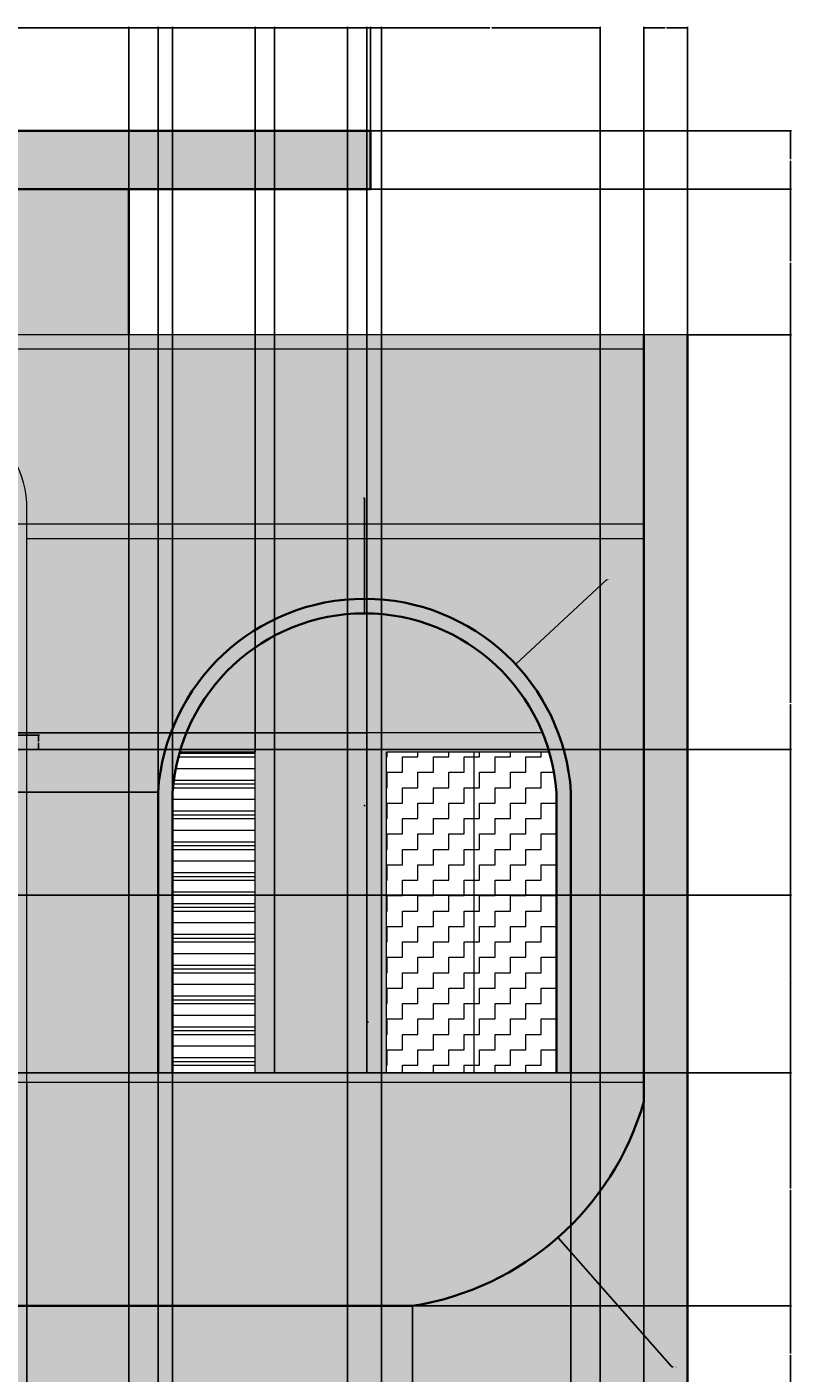
# Model space of a CAD drawing. Units: inches. Extents: x 2051 to 2334, y 814 to 1281.
# Tile 4 of 4: x 2177 to 2334, y 1003 to 1281. Entities that reach past the tile are written whole.
import ezdxf

# ---------------------------------------------------------------- set-up
doc = ezdxf.new("R2010")
doc.units = ezdxf.units.IN
for name, color, linetype, lineweight in [('A-ANNO-DIMS', 2, 'Continuous', 18), ('A-DOOR', 3, 'Continuous', 20), ('A-ELEV-FRAM', 7, 'Continuous', 35), ('A-ELEV-OPEN-PATT', 36, 'Continuous', 13), ('A-ELEV-TRIM', 7, 'Continuous', 18), ('A-ELEV-TRIM-PATT', 7, 'Continuous', 13), ('A-GLAZ', 4, 'Continuous', 18), ('A-GLAZ-PATT', 4, 'Continuous', 13), ('A-ROOF', 7, 'Continuous', 35)]:
    doc.layers.add(name, color=color, linetype=linetype, lineweight=lineweight)
for name, color, linetype, lineweight, true_color in [('A-DOOR-PATT', 251, 'Continuous', 13, 0x636466), ('A-ELEV-FRAM-PATT', 251, 'Continuous', 13, 0x636466), ('A-GLAZ-SCRN-PATT', 251, 'Continuous', 13, 0x636466), ('A-WALL-PATT', 9, 'Continuous', 13, 0xc7c8ca), ('A-WALL-RECS-PATT', 61, 'Continuous', 13, 0xedee99)]:
    doc.layers.add(name, color=color, linetype=linetype, lineweight=lineweight, true_color=true_color)
doc.styles.get("Standard").update_dxf_attribs({"font": 'arial.ttf'})
doc.dimstyles.get("Standard").update_dxf_attribs({"dimtxt": 0.18, "dimasz": 0.18, "dimexe": 0.18, "dimexo": 0.0625, "dimgap": 0.09, "dimtad": 0, "dimtih": 1, "dimtoh": 1, "dimdec": 4, "dimzin": 0, "dimdsep": 46, "dimtxsty": 'Standard', "dimcen": 0.09, "dimadec": 0, "dimazin": 0, "dimtfac": 1, "dimtdec": 4, "dimtofl": 0, "dimtmove": 0, "dimatfit": 3, "dimfxl": 1, "dimtolj": 1, "dimtzin": 0, "dimarcsym": 0})

# ---------------------------------------------------------------- blocks, each defined once
blk = doc.blocks.new('*D6')
at = {"layer": 'A-ANNO-DIMS', "color": 0, "lineweight": -2, "transparency": 16777216}
for p, q in [((2173.99, 1134.81), (2179.51, 1134.81)), ((2179.33, 1134.63), (2179.33, 1133.5)), ((2173.99, 1131.81), (2179.51, 1131.81)), ((2179.33, 1131.99), (2179.33, 1133.13))]:
    blk.add_line(p, q, dxfattribs=at)
at = {"layer": 'A-ANNO-DIMS', "color": 0, "transparency": 16777216}
for points in [[(2179.3, 1134.63), (2179.36, 1134.63), (2179.33, 1134.81)], [(2179.3, 1131.99), (2179.36, 1131.99), (2179.33, 1131.81)]]:
    blk.add_solid(points, dxfattribs=at)
at = {"layer": 'Defpoints', "color": 0, "transparency": 16777216}
for p in [(2173.93, 1134.81), (2179.33, 1134.81), (2173.93, 1131.81)]:
    blk.add_point(p, dxfattribs=at)
at = {"layer": 'A-ANNO-DIMS', "color": 0, "transparency": 16777216, "insert": (2179.33, 1133.31), "char_height": 0.18, "attachment_point": 5}
blk.add_mtext('\\A1;3 TYP.', dxfattribs=at)
blk = doc.blocks.new('*D11')
at = {"layer": 'A-ANNO-DIMS', "color": 0, "lineweight": -2, "transparency": 16777216}
for p, q in [((2256.4, 1017.24), (2334.32, 1017.24)), ((2334.14, 1017.06), (2334.14, 1007.43)), ((2334.14, 997.42), (2334.14, 1007.06)), ((2312.99, 997.24), (2334.32, 997.24))]:
    blk.add_line(p, q, dxfattribs=at)
at = {"layer": 'A-ANNO-DIMS', "color": 0, "transparency": 16777216}
for points in [[(2334.11, 1017.06), (2334.17, 1017.06), (2334.14, 1017.24)], [(2334.11, 997.42), (2334.17, 997.42), (2334.14, 997.24)]]:
    blk.add_solid(points, dxfattribs=at)
at = {"layer": 'Defpoints', "color": 0, "transparency": 16777216}
for p in [(2256.33, 1017.24), (2334.14, 1017.24), (2312.93, 997.24)]:
    blk.add_point(p, dxfattribs=at)
at = {"layer": 'A-ANNO-DIMS', "color": 0, "transparency": 16777216, "insert": (2334.14, 1007.24), "char_height": 0.18, "attachment_point": 5}
blk.add_mtext('\\A1;20', dxfattribs=at)
blk = doc.blocks.new('*D12')
at = {"layer": 'A-ANNO-DIMS', "color": 0, "lineweight": -2, "transparency": 16777216}
for p, q in [((2303.99, 1065.24), (2334.32, 1065.24)), ((2334.14, 1065.06), (2334.14, 1041.43)), ((2334.14, 1017.42), (2334.14, 1041.06)), ((2256.4, 1017.24), (2334.32, 1017.24))]:
    blk.add_line(p, q, dxfattribs=at)
at = {"layer": 'A-ANNO-DIMS', "color": 0, "transparency": 16777216}
for points in [[(2334.11, 1065.06), (2334.17, 1065.06), (2334.14, 1065.24)], [(2334.11, 1017.42), (2334.17, 1017.42), (2334.14, 1017.24)]]:
    blk.add_solid(points, dxfattribs=at)
at = {"layer": 'Defpoints', "color": 0, "transparency": 16777216}
for p in [(2303.93, 1065.24), (2334.14, 1065.24), (2256.33, 1017.24)]:
    blk.add_point(p, dxfattribs=at)
at = {"layer": 'A-ANNO-DIMS', "color": 0, "transparency": 16777216, "insert": (2334.14, 1041.24), "char_height": 0.18, "attachment_point": 5}
blk.add_mtext('\\A1;48', dxfattribs=at)
blk = doc.blocks.new('*D13')
at = {"layer": 'A-ANNO-DIMS', "color": 0, "lineweight": -2, "transparency": 16777216}
for p, q in [((2312.99, 1217.24), (2334.32, 1217.24)), ((2334.14, 1217.06), (2334.14, 1141.43)), ((2334.14, 1065.42), (2334.14, 1141.06)), ((2303.99, 1065.24), (2334.32, 1065.24))]:
    blk.add_line(p, q, dxfattribs=at)
at = {"layer": 'A-ANNO-DIMS', "color": 0, "transparency": 16777216}
for points in [[(2334.11, 1217.06), (2334.17, 1217.06), (2334.14, 1217.24)], [(2334.11, 1065.42), (2334.17, 1065.42), (2334.14, 1065.24)]]:
    blk.add_solid(points, dxfattribs=at)
at = {"layer": 'Defpoints', "color": 0, "transparency": 16777216}
for p in [(2312.93, 1217.24), (2334.14, 1217.24), (2303.93, 1065.24)]:
    blk.add_point(p, dxfattribs=at)
at = {"layer": 'A-ANNO-DIMS', "color": 0, "transparency": 16777216, "insert": (2334.14, 1141.24), "char_height": 0.18, "attachment_point": 5}
blk.add_mtext('\\A1;152', dxfattribs=at)
blk = doc.blocks.new('*D14')
at = {"layer": 'A-ANNO-DIMS', "color": 0, "lineweight": -2, "transparency": 16777216}
for p, q in [((2247.73, 1247.24), (2334.32, 1247.24)), ((2334.14, 1247.06), (2334.14, 1232.43)), ((2334.14, 1217.42), (2334.14, 1232.06)), ((2312.99, 1217.24), (2334.32, 1217.24))]:
    blk.add_line(p, q, dxfattribs=at)
at = {"layer": 'A-ANNO-DIMS', "color": 0, "transparency": 16777216}
for points in [[(2334.11, 1247.06), (2334.17, 1247.06), (2334.14, 1247.24)], [(2334.11, 1217.42), (2334.17, 1217.42), (2334.14, 1217.24)]]:
    blk.add_solid(points, dxfattribs=at)
at = {"layer": 'Defpoints', "color": 0, "transparency": 16777216}
for p in [(2247.66, 1247.24), (2334.14, 1247.24), (2312.93, 1217.24)]:
    blk.add_point(p, dxfattribs=at)
at = {"layer": 'A-ANNO-DIMS', "color": 0, "transparency": 16777216, "insert": (2334.14, 1232.24), "char_height": 0.18, "attachment_point": 5}
blk.add_mtext('\\A1;30', dxfattribs=at)
blk = doc.blocks.new('*D15')
at = {"layer": 'A-ANNO-DIMS', "color": 0, "lineweight": -2, "transparency": 16777216}
for p, q in [((2247.73, 1259.24), (2334.32, 1259.24)), ((2334.14, 1259.06), (2334.14, 1253.42)), ((2334.14, 1247.42), (2334.14, 1253.06)), ((2247.73, 1247.24), (2334.32, 1247.24))]:
    blk.add_line(p, q, dxfattribs=at)
at = {"layer": 'A-ANNO-DIMS', "color": 0, "transparency": 16777216}
for points in [[(2334.11, 1259.06), (2334.17, 1259.06), (2334.14, 1259.24)], [(2334.11, 1247.42), (2334.17, 1247.42), (2334.14, 1247.24)]]:
    blk.add_solid(points, dxfattribs=at)
at = {"layer": 'Defpoints', "color": 0, "transparency": 16777216}
for p in [(2247.66, 1259.24), (2334.14, 1259.24), (2247.66, 1247.24)]:
    blk.add_point(p, dxfattribs=at)
at = {"layer": 'A-ANNO-DIMS', "color": 0, "transparency": 16777216, "insert": (2334.14, 1253.24), "char_height": 0.18, "attachment_point": 5}
blk.add_mtext('\\A1;12', dxfattribs=at)
blk = doc.blocks.new('*D19')
at = {"layer": 'A-ANNO-DIMS', "color": 0, "lineweight": -2, "transparency": 16777216}
for p, q in [((2112.93, 1247.31), (2112.93, 1280.64)), ((2113.11, 1280.46), (2155.21, 1280.46)), ((2197.75, 1280.46), (2155.65, 1280.46)), ((2197.93, 1247.31), (2197.93, 1280.64))]:
    blk.add_line(p, q, dxfattribs=at)
at = {"layer": 'A-ANNO-DIMS', "color": 0, "transparency": 16777216}
for points in [[(2113.11, 1280.49), (2113.11, 1280.43), (2112.93, 1280.46)], [(2197.75, 1280.49), (2197.75, 1280.43), (2197.93, 1280.46)]]:
    blk.add_solid(points, dxfattribs=at)
at = {"layer": 'Defpoints', "color": 0, "transparency": 16777216}
for p in [(2197.93, 1280.46), (2112.93, 1247.24), (2197.93, 1247.24)]:
    blk.add_point(p, dxfattribs=at)
at = {"layer": 'A-ANNO-DIMS', "color": 0, "transparency": 16777216, "insert": (2155.43, 1280.46), "char_height": 0.18, "attachment_point": 5}
blk.add_mtext('\\A1;85', dxfattribs=at)
blk = doc.blocks.new('*D20')
at = {"layer": 'A-ANNO-DIMS', "color": 0, "lineweight": -2, "transparency": 16777216}
for p, q in [((2197.93, 1247.31), (2197.93, 1280.64)), ((2198.11, 1280.46), (2222.4, 1280.46)), ((2247.48, 1280.46), (2223.19, 1280.46)), ((2247.66, 1259.31), (2247.66, 1280.64))]:
    blk.add_line(p, q, dxfattribs=at)
at = {"layer": 'A-ANNO-DIMS', "color": 0, "transparency": 16777216}
for points in [[(2198.11, 1280.49), (2198.11, 1280.43), (2197.93, 1280.46)], [(2247.48, 1280.49), (2247.48, 1280.43), (2247.66, 1280.46)]]:
    blk.add_solid(points, dxfattribs=at)
at = {"layer": 'Defpoints', "color": 0, "transparency": 16777216}
for p in [(2247.66, 1280.46), (2247.66, 1259.24), (2197.93, 1247.24)]:
    blk.add_point(p, dxfattribs=at)
at = {"layer": 'A-ANNO-DIMS', "color": 0, "transparency": 16777216, "insert": (2222.8, 1280.46), "char_height": 0.18, "attachment_point": 5}
blk.add_mtext('\\A1;49.74', dxfattribs=at)
blk = doc.blocks.new('*D21')
at = {"layer": 'A-ANNO-DIMS', "color": 0, "lineweight": -2, "transparency": 16777216}
for p, q in [((2303.93, 1217.31), (2303.93, 1280.64)), ((2304.11, 1280.46), (2308.28, 1280.46)), ((2312.75, 1280.46), (2308.58, 1280.46)), ((2312.93, 1217.31), (2312.93, 1280.64))]:
    blk.add_line(p, q, dxfattribs=at)
at = {"layer": 'A-ANNO-DIMS', "color": 0, "transparency": 16777216}
for points in [[(2304.11, 1280.49), (2304.11, 1280.43), (2303.93, 1280.46)], [(2312.75, 1280.49), (2312.75, 1280.43), (2312.93, 1280.46)]]:
    blk.add_solid(points, dxfattribs=at)
at = {"layer": 'Defpoints', "color": 0, "transparency": 16777216}
for p in [(2312.93, 1280.46), (2303.93, 1217.24), (2312.93, 1217.24)]:
    blk.add_point(p, dxfattribs=at)
at = {"layer": 'A-ANNO-DIMS', "color": 0, "transparency": 16777216, "insert": (2308.43, 1280.46), "char_height": 0.18, "attachment_point": 5}
blk.add_mtext('\\A1;9', dxfattribs=at)
blk = doc.blocks.new('*D22')
at = {"layer": 'A-ANNO-DIMS', "color": 0, "lineweight": -2, "transparency": 16777216}
for p, q in [((2303.93, 1059.18), (2303.93, 813.85)), ((2256.33, 1017.18), (2256.33, 813.85)), ((2256.51, 814.03), (2279.73, 814.03)), ((2303.75, 814.03), (2280.53, 814.03))]:
    blk.add_line(p, q, dxfattribs=at)
at = {"layer": 'A-ANNO-DIMS', "color": 0, "transparency": 16777216}
for points in [[(2256.51, 814.06), (2256.51, 814), (2256.33, 814.03)], [(2303.75, 814.06), (2303.75, 814), (2303.93, 814.03)]]:
    blk.add_solid(points, dxfattribs=at)
at = {"layer": 'Defpoints', "color": 0, "transparency": 16777216}
for p in [(2303.93, 1059.24), (2256.33, 1017.24), (2303.93, 814.03)]:
    blk.add_point(p, dxfattribs=at)
at = {"layer": 'A-ANNO-DIMS', "color": 0, "transparency": 16777216, "insert": (2280.13, 814.03), "char_height": 0.18, "attachment_point": 5}
blk.add_mtext('\\A1;47.59', dxfattribs=at)
blk = doc.blocks.new('*D26')
at = {"layer": 'A-ANNO-DIMS', "color": 0, "lineweight": -2, "transparency": 16777216}
for p, q in [((2203.87, 1123.07), (2051.53, 1123.07)), ((2051.71, 1122.89), (2051.71, 1094.34)), ((2051.71, 1065.42), (2051.71, 1093.98)), ((2203.87, 1065.24), (2051.53, 1065.24))]:
    blk.add_line(p, q, dxfattribs=at)
at = {"layer": 'A-ANNO-DIMS', "color": 0, "transparency": 16777216}
for points in [[(2051.68, 1122.89), (2051.74, 1122.89), (2051.71, 1123.07)], [(2051.68, 1065.42), (2051.74, 1065.42), (2051.71, 1065.24)]]:
    blk.add_solid(points, dxfattribs=at)
at = {"layer": 'Defpoints', "color": 0, "transparency": 16777216}
for p in [(2051.71, 1123.07), (2203.93, 1123.07), (2203.93, 1065.24)]:
    blk.add_point(p, dxfattribs=at)
at = {"layer": 'A-ANNO-DIMS', "color": 0, "transparency": 16777216, "insert": (2051.71, 1094.16), "char_height": 0.18, "attachment_point": 5}
blk.add_mtext('\\A1;57.83', dxfattribs=at)
blk = doc.blocks.new('*D28')
at = {"layer": 'A-ANNO-DIMS', "color": 0, "lineweight": -2, "transparency": 16777216}
for p, q in [((2203.93, 1065.18), (2203.93, 813.85)), ((2176.93, 1063.18), (2176.93, 813.85)), ((2177.11, 814.03), (2190.21, 814.03)), ((2203.75, 814.03), (2190.65, 814.03))]:
    blk.add_line(p, q, dxfattribs=at)
at = {"layer": 'A-ANNO-DIMS', "color": 0, "transparency": 16777216}
for points in [[(2177.11, 814.06), (2177.11, 814), (2176.93, 814.03)], [(2203.75, 814.06), (2203.75, 814), (2203.93, 814.03)]]:
    blk.add_solid(points, dxfattribs=at)
at = {"layer": 'Defpoints', "color": 0, "transparency": 16777216}
for p in [(2203.93, 1065.24), (2176.93, 1063.24), (2203.93, 814.03)]:
    blk.add_point(p, dxfattribs=at)
at = {"layer": 'A-ANNO-DIMS', "color": 0, "transparency": 16777216, "insert": (2190.43, 814.03), "char_height": 0.18, "attachment_point": 5}
blk.add_mtext('\\A1;27', dxfattribs=at)
blk = doc.blocks.new('*D29')
at = {"layer": 'A-ANNO-DIMS', "color": 0, "lineweight": -2, "transparency": 16777216}
for p, q in [((2203.93, 1065.18), (2203.93, 813.85)), ((2288.93, 1065.18), (2288.93, 813.85)), ((2204.11, 814.03), (2246.21, 814.03)), ((2288.75, 814.03), (2246.65, 814.03))]:
    blk.add_line(p, q, dxfattribs=at)
at = {"layer": 'A-ANNO-DIMS', "color": 0, "transparency": 16777216}
for points in [[(2204.11, 814.06), (2204.11, 814), (2203.93, 814.03)], [(2288.75, 814.06), (2288.75, 814), (2288.93, 814.03)]]:
    blk.add_solid(points, dxfattribs=at)
at = {"layer": 'Defpoints', "color": 0, "transparency": 16777216}
for p in [(2203.93, 1065.24), (2288.93, 1065.24), (2288.93, 814.03)]:
    blk.add_point(p, dxfattribs=at)
at = {"layer": 'A-ANNO-DIMS', "color": 0, "transparency": 16777216, "insert": (2246.43, 814.03), "char_height": 0.18, "attachment_point": 5}
blk.add_mtext('\\A1;85', dxfattribs=at)
blk = doc.blocks.new('*D30')
at = {"layer": 'A-ANNO-DIMS', "color": 0, "lineweight": -2, "transparency": 16777216}
for p, q in [((2288.93, 1065.18), (2288.93, 813.85)), ((2303.93, 1065.18), (2303.93, 813.85)), ((2289.11, 814.03), (2296.22, 814.03)), ((2303.75, 814.03), (2296.64, 814.03))]:
    blk.add_line(p, q, dxfattribs=at)
at = {"layer": 'A-ANNO-DIMS', "color": 0, "transparency": 16777216}
for points in [[(2289.11, 814.06), (2289.11, 814), (2288.93, 814.03)], [(2303.75, 814.06), (2303.75, 814), (2303.93, 814.03)]]:
    blk.add_solid(points, dxfattribs=at)
at = {"layer": 'Defpoints', "color": 0, "transparency": 16777216}
for p in [(2288.93, 1065.24), (2303.93, 1065.24), (2303.93, 814.03)]:
    blk.add_point(p, dxfattribs=at)
at = {"layer": 'A-ANNO-DIMS', "color": 0, "transparency": 16777216, "insert": (2296.43, 814.03), "char_height": 0.18, "attachment_point": 5}
blk.add_mtext('\\A1;15', dxfattribs=at)
blk = doc.blocks.new('*D31')
at = {"layer": 'A-ANNO-DIMS', "color": 0, "lineweight": -2, "transparency": 16777216}
for p, q in [((2137.99, 1101.81), (2334.32, 1101.81)), ((2334.14, 1101.63), (2334.14, 1083.71)), ((2334.14, 1065.42), (2334.14, 1083.35)), ((2137.99, 1065.24), (2334.32, 1065.24))]:
    blk.add_line(p, q, dxfattribs=at)
at = {"layer": 'A-ANNO-DIMS', "color": 0, "transparency": 16777216}
for points in [[(2334.11, 1101.63), (2334.17, 1101.63), (2334.14, 1101.81)], [(2334.11, 1065.42), (2334.17, 1065.42), (2334.14, 1065.24)]]:
    blk.add_solid(points, dxfattribs=at)
at = {"layer": 'Defpoints', "color": 0, "transparency": 16777216}
for p in [(2137.93, 1101.81), (2334.14, 1101.81), (2137.93, 1065.24)]:
    blk.add_point(p, dxfattribs=at)
at = {"layer": 'A-ANNO-DIMS', "color": 0, "transparency": 16777216, "insert": (2334.14, 1083.53), "char_height": 0.18, "attachment_point": 5}
blk.add_mtext('\\A1;36.57', dxfattribs=at)
blk = doc.blocks.new('*D32')
at = {"layer": 'A-ANNO-DIMS', "color": 0, "lineweight": -2, "transparency": 16777216}
for p, q in [((2137.99, 1131.81), (2334.32, 1131.81)), ((2334.14, 1131.63), (2334.14, 1117)), ((2334.14, 1101.99), (2334.14, 1116.63)), ((2137.99, 1101.81), (2334.32, 1101.81))]:
    blk.add_line(p, q, dxfattribs=at)
at = {"layer": 'A-ANNO-DIMS', "color": 0, "transparency": 16777216}
for points in [[(2334.11, 1131.63), (2334.17, 1131.63), (2334.14, 1131.81)], [(2334.11, 1101.99), (2334.17, 1101.99), (2334.14, 1101.81)]]:
    blk.add_solid(points, dxfattribs=at)
at = {"layer": 'Defpoints', "color": 0, "transparency": 16777216}
for p in [(2137.93, 1131.81), (2334.14, 1131.81), (2137.93, 1101.81)]:
    blk.add_point(p, dxfattribs=at)
at = {"layer": 'A-ANNO-DIMS', "color": 0, "transparency": 16777216, "insert": (2334.14, 1116.81), "char_height": 0.18, "attachment_point": 5}
blk.add_mtext('\\A1;30', dxfattribs=at)
blk = doc.blocks.new('*D33')
at = {"layer": 'A-ANNO-DIMS', "color": 0, "lineweight": -2, "transparency": 16777216}
for p, q in [((2246.87, 1135.24), (2051.53, 1135.24)), ((2051.71, 1135.06), (2051.71, 1100.43)), ((2051.71, 1065.42), (2051.71, 1100.06)), ((2246.87, 1065.24), (2051.53, 1065.24))]:
    blk.add_line(p, q, dxfattribs=at)
at = {"layer": 'A-ANNO-DIMS', "color": 0, "transparency": 16777216}
for points in [[(2051.68, 1135.06), (2051.74, 1135.06), (2051.71, 1135.24)], [(2051.68, 1065.42), (2051.74, 1065.42), (2051.71, 1065.24)]]:
    blk.add_solid(points, dxfattribs=at)
at = {"layer": 'Defpoints', "color": 0, "transparency": 16777216}
for p in [(2051.71, 1135.24), (2246.93, 1135.24), (2246.93, 1065.24)]:
    blk.add_point(p, dxfattribs=at)
at = {"layer": 'A-ANNO-DIMS', "color": 0, "transparency": 16777216, "insert": (2051.71, 1100.24), "char_height": 0.18, "attachment_point": 5}
blk.add_mtext('\\A1;70', dxfattribs=at)
blk = doc.blocks.new('*D34')
at = {"layer": 'A-ANNO-DIMS', "color": 0, "lineweight": -2, "transparency": 16777216}
for p, q in [((2227.93, 1065.31), (2227.93, 1280.64)), ((2228.11, 1280.46), (2237.22, 1280.46)), ((2246.75, 1280.46), (2237.64, 1280.46)), ((2246.93, 1065.31), (2246.93, 1280.64))]:
    blk.add_line(p, q, dxfattribs=at)
at = {"layer": 'A-ANNO-DIMS', "color": 0, "transparency": 16777216}
for points in [[(2228.11, 1280.49), (2228.11, 1280.43), (2227.93, 1280.46)], [(2246.75, 1280.49), (2246.75, 1280.43), (2246.93, 1280.46)]]:
    blk.add_solid(points, dxfattribs=at)
at = {"layer": 'Defpoints', "color": 0, "transparency": 16777216}
for p in [(2246.93, 1280.46), (2227.93, 1065.24), (2246.93, 1065.24)]:
    blk.add_point(p, dxfattribs=at)
at = {"layer": 'A-ANNO-DIMS', "color": 0, "transparency": 16777216, "insert": (2237.43, 1280.46), "char_height": 0.18, "attachment_point": 5}
blk.add_mtext('\\A1;19', dxfattribs=at)
blk = doc.blocks.new('*D35')
at = {"layer": 'A-ANNO-DIMS', "color": 0, "lineweight": -2, "transparency": 16777216}
for p, q in [((2203.93, 1065.31), (2203.93, 1280.64)), ((2204.11, 1280.46), (2215.71, 1280.46)), ((2227.75, 1280.46), (2216.15, 1280.46)), ((2227.93, 1065.31), (2227.93, 1280.64))]:
    blk.add_line(p, q, dxfattribs=at)
at = {"layer": 'A-ANNO-DIMS', "color": 0, "transparency": 16777216}
for points in [[(2204.11, 1280.49), (2204.11, 1280.43), (2203.93, 1280.46)], [(2227.75, 1280.49), (2227.75, 1280.43), (2227.93, 1280.46)]]:
    blk.add_solid(points, dxfattribs=at)
at = {"layer": 'Defpoints', "color": 0, "transparency": 16777216}
for p in [(2227.93, 1280.46), (2203.93, 1065.24), (2227.93, 1065.24)]:
    blk.add_point(p, dxfattribs=at)
at = {"layer": 'A-ANNO-DIMS', "color": 0, "transparency": 16777216, "insert": (2215.93, 1280.46), "char_height": 0.18, "attachment_point": 5}
blk.add_mtext('\\A1;24', dxfattribs=at)
blk = doc.blocks.new('*D36')
at = {"layer": 'A-ANNO-DIMS', "color": 0, "lineweight": -2, "transparency": 16777216}
for p, q in [((2223.93, 1131.31), (2223.93, 1280.64)), ((2224.11, 1280.46), (2225.78, 1280.46)), ((2227.75, 1280.46), (2226.08, 1280.46)), ((2227.93, 1135.31), (2227.93, 1280.64))]:
    blk.add_line(p, q, dxfattribs=at)
at = {"layer": 'A-ANNO-DIMS', "color": 0, "transparency": 16777216}
for points in [[(2224.11, 1280.49), (2224.11, 1280.43), (2223.93, 1280.46)], [(2227.75, 1280.49), (2227.75, 1280.43), (2227.93, 1280.46)]]:
    blk.add_solid(points, dxfattribs=at)
at = {"layer": 'Defpoints', "color": 0, "transparency": 16777216}
for p in [(2227.93, 1280.46), (2227.93, 1135.24), (2223.93, 1131.24)]:
    blk.add_point(p, dxfattribs=at)
at = {"layer": 'A-ANNO-DIMS', "color": 0, "transparency": 16777216, "insert": (2225.93, 1280.46), "char_height": 0.18, "attachment_point": 5}
blk.add_mtext('\\A1;4', dxfattribs=at)
blk = doc.blocks.new('*D49')
at = {"layer": 'A-ANNO-DIMS', "color": 0, "lineweight": -2, "transparency": 16777216}
for p, q in [((2197.93, 931.31), (2197.93, 1280.64)), ((2198.11, 1280.46), (2202.28, 1280.46)), ((2206.75, 1280.46), (2202.58, 1280.46)), ((2206.93, 946.31), (2206.93, 1280.64))]:
    blk.add_line(p, q, dxfattribs=at)
at = {"layer": 'A-ANNO-DIMS', "color": 0, "transparency": 16777216}
for points in [[(2198.11, 1280.49), (2198.11, 1280.43), (2197.93, 1280.46)], [(2206.75, 1280.49), (2206.75, 1280.43), (2206.93, 1280.46)]]:
    blk.add_solid(points, dxfattribs=at)
at = {"layer": 'Defpoints', "color": 0, "transparency": 16777216}
for p in [(2206.93, 1280.46), (2206.93, 946.24), (2197.93, 931.24)]:
    blk.add_point(p, dxfattribs=at)
at = {"layer": 'A-ANNO-DIMS', "color": 0, "transparency": 16777216, "insert": (2202.43, 1280.46), "char_height": 0.18, "attachment_point": 5}
blk.add_mtext('\\A1;9', dxfattribs=at)
blk = doc.blocks.new('*D50')
at = {"layer": 'A-ANNO-DIMS', "color": 0, "lineweight": -2, "transparency": 16777216}
for p, q in [((2206.93, 946.31), (2206.93, 1280.64)), ((2207.11, 1280.46), (2224.71, 1280.46)), ((2242.75, 1280.46), (2225.15, 1280.46)), ((2242.93, 946.31), (2242.93, 1280.64))]:
    blk.add_line(p, q, dxfattribs=at)
at = {"layer": 'A-ANNO-DIMS', "color": 0, "transparency": 16777216}
for points in [[(2207.11, 1280.49), (2207.11, 1280.43), (2206.93, 1280.46)], [(2242.75, 1280.49), (2242.75, 1280.43), (2242.93, 1280.46)]]:
    blk.add_solid(points, dxfattribs=at)
at = {"layer": 'Defpoints', "color": 0, "transparency": 16777216}
for p in [(2242.93, 1280.46), (2206.93, 946.24), (2242.93, 946.24)]:
    blk.add_point(p, dxfattribs=at)
at = {"layer": 'A-ANNO-DIMS', "color": 0, "transparency": 16777216, "insert": (2224.93, 1280.46), "char_height": 0.18, "attachment_point": 5}
blk.add_mtext('\\A1;36', dxfattribs=at)
blk = doc.blocks.new('*D51')
at = {"layer": 'A-ANNO-DIMS', "color": 0, "lineweight": -2, "transparency": 16777216}
for p, q in [((2242.93, 946.31), (2242.93, 1280.64)), ((2243.11, 1280.46), (2246.28, 1280.46)), ((2249.75, 1280.46), (2246.58, 1280.46)), ((2249.93, 946.31), (2249.93, 1280.64))]:
    blk.add_line(p, q, dxfattribs=at)
at = {"layer": 'A-ANNO-DIMS', "color": 0, "transparency": 16777216}
for points in [[(2243.11, 1280.49), (2243.11, 1280.43), (2242.93, 1280.46)], [(2249.75, 1280.49), (2249.75, 1280.43), (2249.93, 1280.46)]]:
    blk.add_solid(points, dxfattribs=at)
at = {"layer": 'Defpoints', "color": 0, "transparency": 16777216}
for p in [(2249.93, 1280.46), (2242.93, 946.24), (2249.93, 946.24)]:
    blk.add_point(p, dxfattribs=at)
at = {"layer": 'A-ANNO-DIMS', "color": 0, "transparency": 16777216, "insert": (2246.43, 1280.46), "char_height": 0.18, "attachment_point": 5}
blk.add_mtext('\\A1;7', dxfattribs=at)
blk = doc.blocks.new('*D52')
at = {"layer": 'A-ANNO-DIMS', "color": 0, "lineweight": -2, "transparency": 16777216}
for p, q in [((2249.93, 946.31), (2249.93, 1280.64)), ((2250.11, 1280.46), (2272.21, 1280.46)), ((2294.75, 1280.46), (2272.65, 1280.46)), ((2294.93, 946.31), (2294.93, 1280.64))]:
    blk.add_line(p, q, dxfattribs=at)
at = {"layer": 'A-ANNO-DIMS', "color": 0, "transparency": 16777216}
for points in [[(2250.11, 1280.49), (2250.11, 1280.43), (2249.93, 1280.46)], [(2294.75, 1280.49), (2294.75, 1280.43), (2294.93, 1280.46)]]:
    blk.add_solid(points, dxfattribs=at)
at = {"layer": 'Defpoints', "color": 0, "transparency": 16777216}
for p in [(2294.93, 1280.46), (2249.93, 946.24), (2294.93, 946.24)]:
    blk.add_point(p, dxfattribs=at)
at = {"layer": 'A-ANNO-DIMS', "color": 0, "transparency": 16777216, "insert": (2272.43, 1280.46), "char_height": 0.18, "attachment_point": 5}
blk.add_mtext('\\A1;45', dxfattribs=at)
blk = doc.blocks.new('*D54')
at = {"layer": 'A-ANNO-DIMS', "color": 0, "lineweight": -2, "transparency": 16777216}
for p, q in [((2246.99, 1075.7), (2247.17, 1075.7)), ((2247.08, 1075.61), (2247.08, 1075.79)), ((2309.73, 1004.7), (2286.36, 1031.19)), ((2309.91, 1004.7), (2309.73, 1004.7))]:
    blk.add_line(p, q, dxfattribs=at)
at = {"layer": 'A-ANNO-DIMS', "color": 0, "transparency": 16777216}
blk.add_solid([(2286.38, 1031.21), (2286.34, 1031.17), (2286.24, 1031.32)], dxfattribs=at)
at = {"layer": 'Defpoints', "color": 0, "transparency": 16777216}
for p in [(2247.08, 1075.7), (2286.24, 1031.32)]:
    blk.add_point(p, dxfattribs=at)
at = {"layer": 'A-ANNO-DIMS', "color": 0, "transparency": 16777216, "insert": (2310.39, 1004.7), "char_height": 0.18, "attachment_point": 5}
blk.add_mtext('\\A1;R59.18', dxfattribs=at)
blk = doc.blocks.new('*D57')
at = {"layer": 'A-ANNO-DIMS', "color": 0, "lineweight": -2, "transparency": 16777216}
for p, q in [((2296.22, 1166.8), (2277.68, 1149.47)), ((2296.4, 1166.8), (2296.22, 1166.8)), ((2246.34, 1120.27), (2246.52, 1120.27)), ((2246.43, 1120.18), (2246.43, 1120.36))]:
    blk.add_line(p, q, dxfattribs=at)
at = {"layer": 'A-ANNO-DIMS', "color": 0, "transparency": 16777216}
blk.add_solid([(2277.66, 1149.5), (2277.7, 1149.45), (2277.55, 1149.35)], dxfattribs=at)
at = {"layer": 'Defpoints', "color": 0, "transparency": 16777216}
for p in [(2277.55, 1149.35), (2246.43, 1120.27)]:
    blk.add_point(p, dxfattribs=at)
at = {"layer": 'A-ANNO-DIMS', "color": 0, "transparency": 16777216, "insert": (2296.88, 1166.8), "char_height": 0.18, "attachment_point": 5}
blk.add_mtext('\\A1;R42.59', dxfattribs=at)
blk = doc.blocks.new('*D58')
at = {"layer": 'A-ANNO-DIMS', "color": 0, "lineweight": -2, "transparency": 16777216}
for p, q in [((2246.25, 1183.62), (2246.43, 1183.62)), ((2246.43, 1183.62), (2246.43, 1160.05)), ((2246.34, 1120.27), (2246.52, 1120.27)), ((2246.43, 1120.18), (2246.43, 1120.36))]:
    blk.add_line(p, q, dxfattribs=at)
at = {"layer": 'A-ANNO-DIMS', "color": 0, "transparency": 16777216}
blk.add_solid([(2246.46, 1160.05), (2246.4, 1160.05), (2246.43, 1159.87)], dxfattribs=at)
at = {"layer": 'Defpoints', "color": 0, "transparency": 16777216}
for p in [(2246.43, 1159.87), (2246.43, 1120.27)]:
    blk.add_point(p, dxfattribs=at)
at = {"layer": 'A-ANNO-DIMS', "color": 0, "transparency": 16777216, "insert": (2245.77, 1183.62), "char_height": 0.18, "attachment_point": 5}
blk.add_mtext('\\A1;R39.59', dxfattribs=at)

msp = doc.modelspace()

# ---------------------------------------------------------------- hatches: boundary and pattern name
at = {"layer": 'A-DOOR-PATT', "transparency": 33554595}
h = msp.add_hatch(dxfattribs=at)
h.set_pattern_fill('ZIGZAG', color=256)
h.set_pattern_definition([(0, (0, 0), (3.175, 3.175), [3.175, -3.175]), (90, (3.175, 0), (-3.175, 3.175), [3.175, -3.175])])
h.paths.add_polyline_path([(2285.9283, 1122.9709, 0.05319425), (2284.4701, 1131.2439), (2268.9283, 1131.2439), (2268.9283, 1065.2439), (2285.9283, 1065.2439)])
h.paths.add_polyline_path([(2268.9283, 1131.2439), (2250.9283, 1131.2439), (2250.9283, 1065.2439), (2268.9283, 1065.2439)])
h.paths.add_polyline_path([(2272.4283, 943.2439), (2252.9283, 943.2439), (2252.9283, 931.2439), (2272.4283, 931.2439)])
h.paths.add_polyline_path([(2291.9283, 943.2439), (2272.4283, 943.2439), (2272.4283, 931.2439), (2291.9283, 931.2439)])
at = {"layer": 'A-ELEV-FRAM-PATT'}
h = msp.add_hatch(color=256, dxfattribs=at)
h.dxf.hatch_style = 1
h.paths.add_polyline_path([(2312.9283, 1217.2439), (2303.9283, 1217.2439), (2303.9283, 1059.2439, -0.29083376), (2256.3338, 1017.2439), (2110.9283, 1017.2439, -0.41949346), (2084.9283, 1039.0559), (2084.9283, 1221.9535, -0.37464242), (2110.9283, 1247.2439), (2247.6639, 1247.2439), (2247.6639, 1259.2439), (2072.9283, 1259.2439), (2072.9283, 835.2439), (2084.9283, 835.2439), (2084.9283, 967.2832, -0.36016597), (2115.4224, 997.2439), (2312.9283, 997.2439)])
h = msp.add_hatch(color=256, dxfattribs=at)
h.dxf.hatch_style = 1
h.paths.add_polyline_path([(2206.9283, 1122.9709, -0.93403721), (2285.9283, 1122.9709), (2285.9283, 1065.2439), (2288.9283, 1065.2439), (2288.9283, 1123.0714, 0.93632991), (2203.9283, 1123.0714), (2203.9283, 1065.2439), (2206.9283, 1065.2439)])
at = {"layer": 'A-ELEV-OPEN-PATT'}
h = msp.add_hatch(color=256, dxfattribs=at)
h.dxf.hatch_style = 1
h.paths.add_polyline_path([(2227.9283, 1135.2439), (2209.7757, 1135.2439, 0.02675663), (2208.3865, 1131.2439), (2223.9283, 1131.2439), (2223.9283, 1065.2439), (2227.9283, 1065.2439)])
h.paths.add_polyline_path([(2250.9283, 1131.2439), (2284.4701, 1131.2439, 0.02675663), (2283.0809, 1135.2439), (2246.9283, 1135.2439), (2246.9283, 1065.2439), (2250.9283, 1065.2439)])
h.paths.add_polyline_path([(2242.9283, 946.2439), (2206.9283, 946.2439), (2206.9283, 931.2439), (2209.9283, 931.2439), (2209.9283, 943.2439), (2239.9283, 943.2439), (2239.9283, 931.2439), (2242.9283, 931.2439)])
h.paths.add_polyline_path([(2252.9283, 943.2439), (2291.9283, 943.2439), (2291.9283, 931.2439), (2294.9283, 931.2439), (2294.9283, 946.2439), (2249.9283, 946.2439), (2249.9283, 931.2439), (2252.9283, 931.2439)])
at = {"layer": 'A-ELEV-TRIM-PATT'}
h = msp.add_hatch(color=256, dxfattribs=at)
h.dxf.hatch_style = 1
h.paths.add_polyline_path([(2098.9283, 1243.754, 0.02131102), (2096.9283, 1242.5167), (2096.9283, 1020.2168, 0.02356469), (2098.9283, 1019.2065)])
h.paths.add_polyline_path([(2303.9283, 1217.2439), (2112.9283, 1217.2439), (2112.9283, 1214.2439), (2303.9283, 1214.2439)])
h.paths.add_polyline_path([(2303.9283, 1178.2439), (2176.9283, 1178.2439), (2176.9283, 1175.2439), (2303.9283, 1175.2439)])
h.paths.add_polyline_path([(2176.9283, 1182.698, 0.9311192), (2134.9283, 1182.698), (2134.9283, 1063.2439), (2176.9283, 1063.2439)])
h.paths.add_polyline_path([(2173.9283, 1065.2439), (2137.9283, 1065.2439), (2137.9283, 1182.698), (2137.9372, 1182.698, -0.9229497), (2173.9283, 1182.5869)], flags=16)
h = msp.add_hatch(color=256, dxfattribs=at)
h.dxf.hatch_style = 1
h.paths.add_polyline_path([(2303.9283, 1065.2439), (2176.9283, 1065.2439), (2176.9283, 1063.2439), (2303.9283, 1063.2439)])
at = {"layer": 'A-GLAZ-PATT', "transparency": 33554595}
h = msp.add_hatch(color=256, dxfattribs=at)
h.dxf.hatch_style = 1
h.set_gradient(color1=(255, 255, 255), color2=(0, 255, 255), name='INVCURVED')
h.paths.add_polyline_path([(2303.9283, 1214.2439), (2112.9283, 1214.2439), (2112.9283, 1178.2439), (2134.9283, 1178.2439), (2134.9283, 1182.698, -0.9311192), (2176.9283, 1182.698), (2176.9283, 1178.2439), (2303.9283, 1178.2439)])
h = msp.add_hatch(color=256, dxfattribs=at)
h.dxf.hatch_style = 1
h.set_gradient(color1=(255, 255, 255), color2=(0, 255, 255), name='INVCURVED')
h.paths.add_polyline_path([(2303.9283, 1059.2439), (2303.9283, 1063.2439), (2112.9283, 1063.2439), (2112.9283, 1017.2439), (2256.3338, 1017.2439, 0.29083376)])
at = {"layer": 'A-GLAZ-SCRN-PATT', "transparency": 33554595}
h = msp.add_hatch(dxfattribs=at)
h.set_pattern_fill('PLASTI', color=256)
h.paths.add_polyline_path([(2223.9283, 1131.2439), (2208.3865, 1131.2439, 0.05319425), (2206.9283, 1122.9709), (2206.9283, 1065.2439), (2223.9283, 1065.2439)])
h.paths.add_polyline_path([(2239.9283, 943.2439), (2224.9283, 943.2439), (2224.9283, 931.2439), (2239.9283, 931.2439)])
h.paths.add_polyline_path([(2224.9283, 943.2439), (2209.9283, 943.2439), (2209.9283, 931.2439), (2224.9283, 931.2439)])
at = {"layer": 'A-WALL-PATT'}
h = msp.add_hatch(color=256, dxfattribs=at)
h.dxf.hatch_style = 1
h.paths.add_polyline_path([(2188.9283, 910.0037, 0.33864929), (2153.1397, 937.3832), (2125.034, 937.3832), (2125.034, 859.2439), (2188.9283, 859.2439)])
h.paths.add_polyline_path([(2113.034, 937.3832), (2084.9283, 937.3832), (2084.9283, 859.2439), (2113.034, 859.2439)])
h.paths.add_polyline_path([(2312.9283, 859.2439), (2084.9283, 859.2439), (2084.9283, 835.2439), (2312.9283, 835.2439)])
h.paths.add_polyline_path([(2288.9283, 1123.0714), (2288.9283, 1065.2439), (2303.9283, 1065.2439), (2303.9283, 1175.2439), (2176.9283, 1175.2439), (2176.9283, 1065.2439), (2203.9283, 1065.2439), (2203.9283, 1123.0714, -0.93632991)])
h.paths.add_polyline_path([(2197.9283, 1247.2439), (2112.9283, 1247.2439), (2112.9283, 1217.2439), (2197.9283, 1217.2439)])
h.paths.add_polyline_path([(2110.9283, 1247.2439, 0.11468321), (2098.9283, 1243.754), (2098.9283, 1019.2065, 0.12996728), (2110.9283, 1017.2439)])
h.paths.add_polyline_path([(2096.9283, 1242.5167, 0.22673474), (2084.9283, 1221.9535), (2084.9283, 1039.0559, 0.24937907), (2096.9283, 1020.2168)])
at = {"layer": 'A-WALL-RECS-PATT'}
h = msp.add_hatch(color=256, dxfattribs=at)
h.dxf.hatch_style = 1
h.paths.add_polyline_path([(2246.9283, 1135.2439), (2283.0809, 1135.2439, 0.67175394), (2209.7757, 1135.2439), (2227.9283, 1135.2439), (2227.9283, 1065.2439), (2246.9283, 1065.2439)])

# ---------------------------------------------------------------- linework, layer by layer
at = {"layer": 'A-DOOR'}
for p, q in [((2246.9283, 1065.2439), (2246.9283, 1135.2439)), ((2283.0809, 1135.2439), (2246.9283, 1135.2439)), ((2284.4701, 1131.2439), (2250.9283, 1131.2439)), ((2250.9283, 1065.2439), (2250.9283, 1131.2439)), ((2268.9283, 1131.2439), (2268.9283, 1065.2439))]:
    msp.add_line(p, q, dxfattribs=at)
at = {"layer": 'A-ELEV-FRAM'}
for p, q in [((2303.9283, 1059.2439), (2303.9283, 1217.2439)), ((2312.9283, 835.2439), (2312.9283, 1217.2439)), ((2256.3338, 1017.2439), (2106.3513, 1017.2439))]:
    msp.add_line(p, q, dxfattribs=at)
for points in [[(2288.9283, 1065.2439), (2288.9283, 1123.0714, 0.93632991), (2203.9283, 1123.0714), (2203.9283, 1065.2439)], [(2285.9283, 1065.2439), (2285.9283, 1122.9709, 0.93403721), (2206.9283, 1122.9709), (2206.9283, 1065.2439)]]:
    msp.add_lwpolyline(points, format="xyb", dxfattribs=at)
msp.add_arc((2247.0817, 1075.6955), 59.1793, 278.994519, 343.859376, dxfattribs=at)
at = {"layer": 'A-ELEV-TRIM'}
for p, q in [((2312.9283, 1217.2439), (2112.9283, 1217.2439)), ((2303.9283, 1214.2439), (2112.9283, 1214.2439)), ((2303.9283, 1178.2439), (2173.9283, 1178.2439)), ((2303.9283, 1175.2439), (2176.9283, 1175.2439)), ((2303.9283, 1065.2439), (2176.9283, 1065.2439)), ((2303.9283, 1063.2439), (2134.9283, 1063.2439))]:
    msp.add_line(p, q, dxfattribs=at)
at = {"layer": 'A-GLAZ'}
for p, q in [((2176.9283, 1063.2439), (2176.9283, 1182.698)), ((2227.9283, 1135.2439), (2209.7757, 1135.2439)), ((2227.9283, 1065.2439), (2227.9283, 1135.2439)), ((2223.9283, 1131.2439), (2208.3865, 1131.2439)), ((2223.9283, 1065.2439), (2223.9283, 1131.2439))]:
    msp.add_line(p, q, dxfattribs=at)
msp.add_arc((2155.9283, 1181.198), 21.0535, 4.085617, 184.085617, dxfattribs=at)
at = {"layer": 'A-ROOF'}
for p, q in [((2247.6639, 1259.2439), (2072.9283, 1259.2439)), ((2247.6639, 1247.2439), (2247.6639, 1259.2439)), ((2247.6639, 1247.2439), (2110.9283, 1247.2439)), ((2197.9283, 1217.2439), (2197.9283, 1247.2439))]:
    msp.add_line(p, q, dxfattribs=at)

# ---------------------------------------------------------------- dimensions: what is measured, and where the dimension line sits
at = {"layer": 'A-ANNO-DIMS'}
for base, p1, p2, override, picture, middle in [((2197.9283, 1280.4589), (2112.9283, 1247.2439), (2197.9283, 1247.2439), {"dimdec": 0, "dimlfac": 1, "dimrnd": 0, "dimzin": 0, "dimdsep": 46, "dimlunit": 2}, '*D19', (2155.4283, 1280.4589)), ((2247.6639, 1280.4589), (2197.9283, 1247.2439), (2247.6639, 1259.2439), {"dimdec": 2, "dimlfac": 1, "dimrnd": 0, "dimzin": 0, "dimdsep": 46, "dimlunit": 2}, '*D20', (2222.7961, 1280.4589)), ((2206.9283, 1280.4589), (2197.9283, 931.2439), (2206.9283, 946.2439), {"dimdec": 0, "dimlfac": 1, "dimrnd": 0, "dimzin": 0, "dimdsep": 46, "dimlunit": 2}, '*D49', (2202.4283, 1280.4589)), ((2227.9283, 1280.4589), (2203.9283, 1065.2439), (2227.9283, 1065.2439), {"dimdec": 0, "dimlfac": 1, "dimrnd": 0, "dimzin": 0, "dimdsep": 46, "dimlunit": 2}, '*D35', (2215.9283, 1280.4589)), ((2242.9283, 1280.4589), (2206.9283, 946.2439), (2242.9283, 946.2439), {"dimdec": 0, "dimlfac": 1, "dimrnd": 0, "dimzin": 0, "dimdsep": 46, "dimlunit": 2}, '*D50', (2224.9283, 1280.4589)), ((2227.9283, 1280.4589), (2223.9283, 1131.2439), (2227.9283, 1135.2439), {"dimdec": 0, "dimlfac": 1, "dimrnd": 0, "dimzin": 0, "dimdsep": 46, "dimlunit": 2}, '*D36', (2225.9283, 1280.4589)), ((2246.9283, 1280.4589), (2227.9283, 1065.2439), (2246.9283, 1065.2439), {"dimdec": 0, "dimlfac": 1, "dimrnd": 0, "dimzin": 0, "dimdsep": 46, "dimlunit": 2}, '*D34', (2237.4283, 1280.4589)), ((2249.9283, 1280.4589), (2242.9283, 946.2439), (2249.9283, 946.2439), {"dimdec": 0, "dimlfac": 1, "dimrnd": 0, "dimzin": 0, "dimdsep": 46, "dimlunit": 2}, '*D51', (2246.4283, 1280.4589)), ((2294.9283, 1280.4589), (2249.9283, 946.2439), (2294.9283, 946.2439), {"dimdec": 0, "dimlfac": 1, "dimrnd": 0, "dimzin": 0, "dimdsep": 46, "dimlunit": 2}, '*D52', (2272.4283, 1280.4589)), ((2312.9283, 1280.4589), (2303.9283, 1217.2439), (2312.9283, 1217.2439), {"dimdec": 0, "dimlfac": 1, "dimrnd": 0, "dimzin": 0, "dimdsep": 46, "dimlunit": 2}, '*D21', (2308.4283, 1280.4589)), ((2203.9283, 814.0289), (2176.9283, 1063.2439), (2203.9283, 1065.2439), {"dimdec": 0, "dimlfac": 1, "dimrnd": 0, "dimzin": 0, "dimdsep": 46, "dimlunit": 2}, '*D28', (2190.4283, 814.0289)), ((2288.9283, 814.0289), (2203.9283, 1065.2439), (2288.9283, 1065.2439), {"dimdec": 0, "dimlfac": 1, "dimrnd": 0, "dimzin": 0, "dimdsep": 46, "dimlunit": 2}, '*D29', (2246.4283, 814.0289)), ((2303.9283, 814.0289), (2288.9283, 1065.2439), (2303.9283, 1065.2439), {"dimdec": 0, "dimlfac": 1, "dimrnd": 0, "dimzin": 0, "dimdsep": 46, "dimlunit": 2}, '*D30', (2296.4283, 814.0289)), ((2303.9283, 814.0289), (2256.3338, 1017.2439), (2303.9283, 1059.2439), {"dimdec": 2, "dimlfac": 1, "dimrnd": 0, "dimzin": 0, "dimdsep": 46, "dimlunit": 2}, '*D22', (2280.131, 814.0289))]:
    dim = msp.add_linear_dim(base=base, p1=p1, p2=p2, dimstyle='Standard', override=override, dxfattribs=at)
    dim.commit()
    dim.dimension.update_dxf_attribs({"geometry": picture, "text_midpoint": middle})
for base, p1, p2, override, picture, middle in [((2334.1433, 1259.2439), (2247.6639, 1247.2439), (2247.6639, 1259.2439), {"dimdec": 0, "dimlfac": 1, "dimrnd": 0, "dimzin": 0, "dimdsep": 46, "dimlunit": 2}, '*D15', (2334.1433, 1253.2439)), ((2334.1433, 1247.2439), (2312.9283, 1217.2439), (2247.6639, 1247.2439), {"dimdec": 0, "dimlfac": 1, "dimrnd": 0, "dimzin": 0, "dimdsep": 46, "dimlunit": 2}, '*D14', (2334.1433, 1232.2439)), ((2334.1433, 1217.2439), (2303.9283, 1065.2439), (2312.9283, 1217.2439), {"dimdec": 0, "dimlfac": 1, "dimrnd": 0, "dimzin": 0, "dimdsep": 46, "dimlunit": 2}, '*D13', (2334.1433, 1141.2439)), ((2051.7133, 1135.2439), (2246.9283, 1065.2439), (2246.9283, 1135.2439), {"dimdec": 0, "dimlfac": 1, "dimrnd": 0, "dimzin": 0, "dimdsep": 46, "dimlunit": 2}, '*D33', (2051.7133, 1100.2439)), ((2334.1433, 1131.8149), (2137.9283, 1101.8149), (2137.9283, 1131.8149), {"dimdec": 0, "dimlfac": 1, "dimrnd": 0, "dimzin": 0, "dimdsep": 46, "dimlunit": 2}, '*D32', (2334.1433, 1116.8149)), ((2051.7133, 1123.0714), (2203.9283, 1065.2439), (2203.9283, 1123.0714), {"dimdec": 2, "dimlfac": 1, "dimrnd": 0, "dimzin": 0, "dimdsep": 46, "dimlunit": 2}, '*D26', (2051.7133, 1094.1576)), ((2334.1433, 1101.8149), (2137.9283, 1065.2439), (2137.9283, 1101.8149), {"dimdec": 2, "dimlfac": 1, "dimrnd": 0, "dimzin": 0, "dimdsep": 46, "dimlunit": 2}, '*D31', (2334.1433, 1083.5294)), ((2334.1433, 1065.2439), (2256.3338, 1017.2439), (2303.9283, 1065.2439), {"dimdec": 0, "dimlfac": 1, "dimrnd": 0, "dimzin": 0, "dimdsep": 46, "dimlunit": 2}, '*D12', (2334.1433, 1041.2439)), ((2334.1433, 1017.2439), (2312.9283, 997.2439), (2256.3338, 1017.2439), {"dimdec": 0, "dimlfac": 1, "dimrnd": 0, "dimzin": 0, "dimdsep": 46, "dimlunit": 2}, '*D11', (2334.1433, 1007.2439))]:
    dim = msp.add_linear_dim(base=base, p1=p1, p2=p2, angle=90, dimstyle='Standard', override=override, dxfattribs=at)
    dim.commit()
    dim.dimension.update_dxf_attribs({"geometry": picture, "text_midpoint": middle})
for center, mpoint, picture, middle in [((2246.4283, 1120.2734), (2246.428, 1159.8654), '*D58', (2245.7678, 1183.6206)), ((2246.4283, 1120.2734), (2277.5506, 1149.3506), '*D57', (2296.884, 1166.7969)), ((2247.0817, 1075.6955), (2286.2389, 1031.3231), '*D54', (2310.3932, 1004.6997))]:
    dim = msp.add_radius_dim(center=center, mpoint=mpoint, dimstyle='Standard', override={"dimdec": 2, "dimlfac": 1, "dimrnd": 0, "dimzin": 0, "dimdsep": 46, "dimlunit": 2}, dxfattribs=at)
    dim.commit()
    dim.dimension.update_dxf_attribs({"geometry": picture, "text_midpoint": middle, "dimtype": 164})
dim = msp.add_linear_dim(base=(2179.3283, 1134.8149), p1=(2173.9283, 1131.8149), p2=(2173.9283, 1134.8149), angle=90, text='<> TYP.', dimstyle='Standard', override={"dimdec": 0, "dimlfac": 1, "dimrnd": 0, "dimzin": 0, "dimdsep": 46, "dimlunit": 2}, dxfattribs=at)
dim.commit()
dim.dimension.update_dxf_attribs({"geometry": '*D6', "text_midpoint": (2179.3283, 1133.3149)})

doc.saveas('drawing.dxf')
